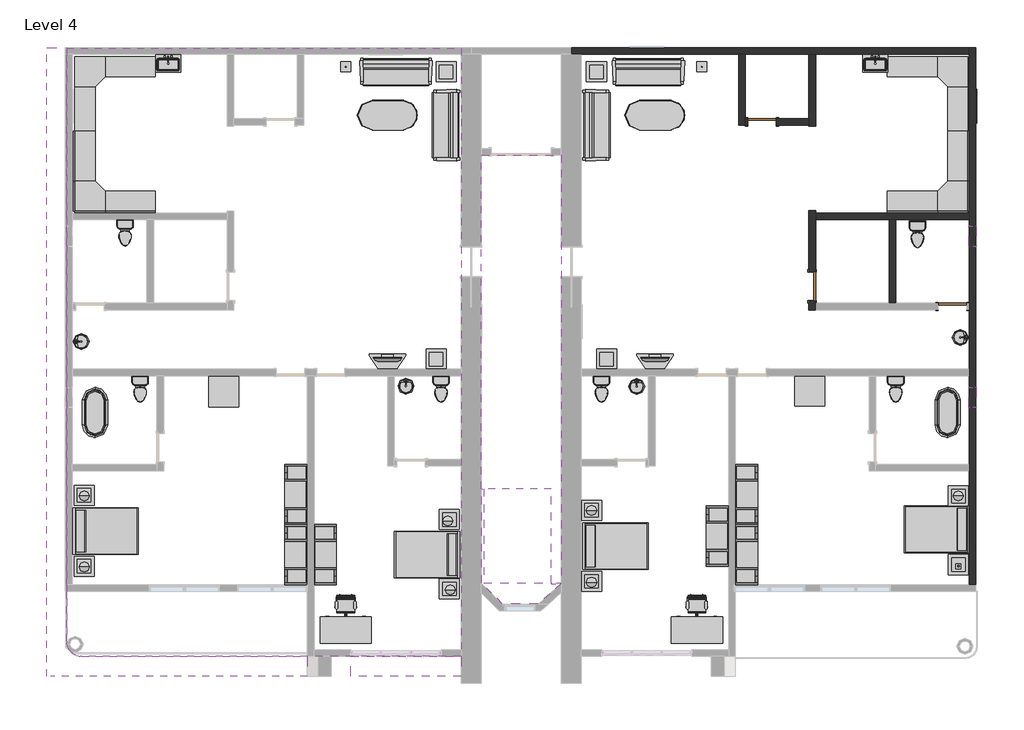
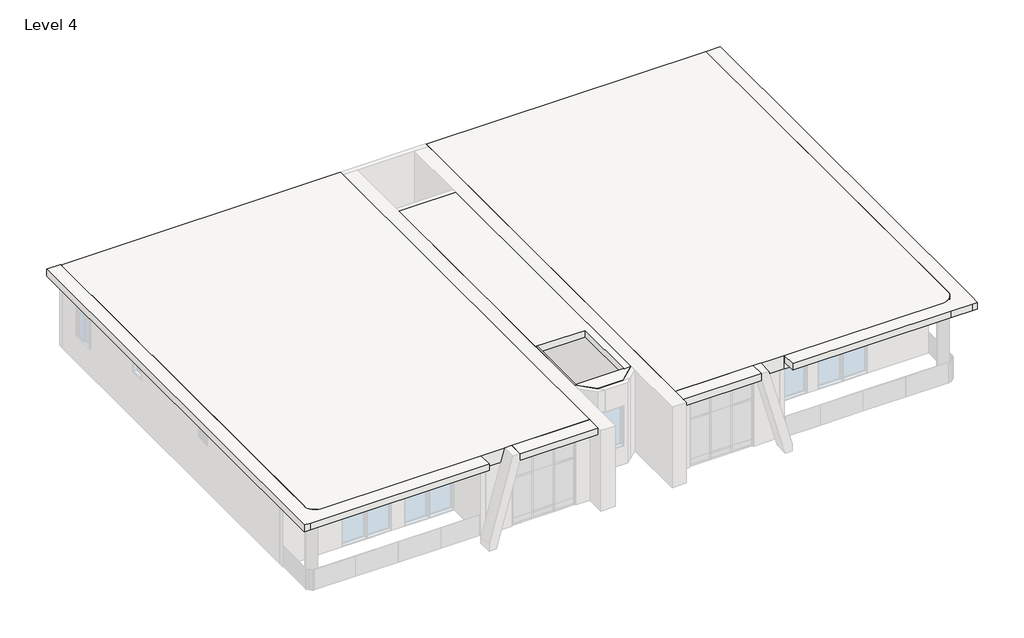
# One storey, part 3 of 3: 42 furniture elements, 14 flow terminals, 10 light fixtures, 8 walls, 5 slabs, 3 doors, 3 windows.
# Revit data of these elements (continued)
# Elements 42, 43, 44, 45, 46, 47, 48, 49, 50, 51, 52, 53 (IfcFurniture, "Table-Coffee : 24\" x 24\" x 24\"")
#   Phase Created = New Construction
#   Materials on its faces: "Glass - Clear, Grey"
# Elements 54, 55 (IfcFurniture, "Table-Dining Oval : 36\" x 72\"")
#   Phase Created = New Construction
#   Materials on its faces: "Steel, Chrome Plated", "Glass - Clear, Grey"
# Elements 56, 57 (IfcFurniture, "Table-Rectangular : 36\" x 36\"")
#   Phase Created = New Construction
#   Materials on its faces: "Birch"
# Elements 58, 59 (IfcFurniture, "Work Station Cubicle : 96\" x 96\"")
#   Phase Created = New Construction
#   Materials on its faces: "Textile - Light Gray", "Laminate, Ivory, Matte"
# Element 60 (IfcLightFixture, "100W - 120V")
#   Mark = "54"
#   Phase Created = New Construction
#   Materials on its faces: "Steel, Chrome Plated", "Glass, Frosted"
# Element 61 (IfcLightFixture, "100W - 120V")
#   Mark = "55"
#   Phase Created = New Construction
#   Materials on its faces: "Steel, Chrome Plated", "Glass, Frosted"
# Element 62 (IfcLightFixture, "Table Lamp - Hemispheric : 60W - 120V")
#   Mark = "56"
#   Phase Created = New Construction
#   Materials on its faces: "Steel, Chrome Plated", "Glass, Frosted", "Birch"
# Element 63 (IfcLightFixture, "Table Lamp - Hemispheric : 60W - 120V")
#   Mark = "57"
#   Phase Created = New Construction
#   Materials on its faces: "Steel, Chrome Plated", "Glass, Frosted", "Birch"
# Element 64 (IfcLightFixture, "Table Lamp - Hemispheric : 60W - 120V")
#   Mark = "58"
#   Phase Created = New Construction
#   Materials on its faces: "Steel, Chrome Plated", "Glass, Frosted", "Birch"
# Element 65 (IfcLightFixture, "Table Lamp - Hemispheric : 60W - 120V")
#   Mark = "59"
#   Phase Created = New Construction
#   Materials on its faces: "Steel, Chrome Plated", "Glass, Frosted", "Birch"
# Element 66 (IfcLightFixture, "Table Lamp - Hemispheric : 60W - 120V")
#   Mark = "60"
#   Phase Created = New Construction
#   Materials on its faces: "Steel, Chrome Plated", "Glass, Frosted", "Birch"
# Element 67 (IfcLightFixture, "Table Lamp - Hemispheric : 60W - 120V")
#   Mark = "61"
#   Phase Created = New Construction
#   Materials on its faces: "Steel, Chrome Plated", "Glass, Frosted", "Birch"
# Element 68 (IfcLightFixture, "Table Lamp - Hemispheric : 60W - 120V")
#   Mark = "62"
#   Phase Created = New Construction
#   Materials on its faces: "Steel, Chrome Plated", "Glass, Frosted", "Birch"
# Element 69 (IfcLightFixture, "Table Lamp - Hemispheric : 60W - 120V")
#   Mark = "63"
#   Phase Created = New Construction
#   Materials on its faces: "Steel, Chrome Plated", "Glass, Frosted", "Birch"
# Element 70 (IfcSlab, "Generic - 12\" cream")
#   Height Offset From Level = 12' - 0"
#   Phase Created = New Construction
#   Materials on its faces: "Parking Stripe"
# Element 71 (IfcSlab, "Generic - 12\" white")
#   built-in parameter 1001955 = 3.14159 (stored number, unit not read)
#   Height Offset From Level = 12' - 0"
#   Phase Created = New Construction
#   Materials on its faces: "Door - Frame"
# Elements 72, 73, 74 (IfcSlab, "Generic - 12\" white")
#   Height Offset From Level = 12' - 0"
#   Phase Created = New Construction
#   Materials on its faces: "Door - Frame"
# Elements 75, 76, 77, 78, 79, 80, 81 (IfcWall, "Generic - 8\" cream")
#   Top Offset = 0' - 0"
#   Base Offset = 0' - 0"
#   Unconnected Height = 10' - 0"
#   wall height = 10' - 0"
#   Phase Created = New Construction
#   Base Constraint = Level 4
#   Materials on its faces: "Parking Stripe"
# Element 82 (IfcWall, "Generic - 8\" white")
#   Top Offset = 0' - 0"
#   Base Offset = 0' - 0"
#   Unconnected Height = 10' - 0"
#   wall height = 10' - 0"
#   Phase Created = New Construction
#   Base Constraint = Level 4
#   Materials on its faces: "Door - Frame", "Parking Stripe"
# Element 83 (IfcWindow, "Louvers with Trim : 24\" x 24\"")
#   Mark = "110"
#   Phase Created = New Construction
#   Materials on its faces: "Glass", "Iron, Ductile"
# Element 84 (IfcWindow, "Louvers with Trim : 24\" x 24\"")
#   Mark = "111"
#   Phase Created = New Construction
#   Materials on its faces: "Glass", "Iron, Ductile"
# Element 85 (IfcWindow, "Slider with Trim : 36\" x 48\"")
#   Mark = "107"
#   Phase Created = New Construction
#   Materials on its faces: "Iron, Ductile", "Glass"
# Materials
#   "Wood - Birch - Solid Stained Light Low Gloss": class "Wood", colour RGB 210 159 95, transparency 0, Cost = 0
#   "Paint - Sienna": colour RGB 118 70 51, transparency 0, Cost = 0
#   "Steel, Polished": class "Metal", colour RGB 57 57 57, transparency 0, Description = "Polished steel", Cost = 0
#   "Porcelain, Linen": class "Ceramic", colour RGB 249 239 230, transparency 0, Description = "Porcelain, linen", Cost = 0
#   "Laminate, Linen, Matte": class "Plastic", colour RGB 249 239 230, transparency 0, Description = "Plastic Laminate - Linen, Matte", Cost = 0
#   "Porcelain, Ivory": class "Ceramic", colour RGB 247 247 239, transparency 0, Description = "Porcelain, ivory", Cost = 0
#   "Laminate, Ivory, Matte": class "Plastic", colour RGB 247 247 239, transparency 0, Description = "Plastic Laminate - Ivory, Matte", Cost = 0
#   "Birch": class "Wood", colour RGB 224 178 126, transparency 0, Description = "Betula Alleghaniensis", Cost = 0
#   "Linen, White": class "Textile", colour RGB 247 247 239, transparency 0, Description = "Linen, white", Cost = 0
#   "Plastic, Opaque Black": class "Plastic", colour RGB 0 0 0, transparency 0.7, Description = "Plastic, generic, opaque black", Cost = 0
#   "Textile - Slate Blue": class "Fabric", colour RGB 98 102 118, transparency 0
#   "Steel, Chrome Plated": class "Metal", colour RGB 17 17 17, transparency 0, Description = "Chromiuim plated steel", Cost = 0
#   "Cherry": class "Wood", colour RGB 226 177 128, transparency 0, Description = "Prunus Serotina", Cost = 0
#   "Linen, Beige": class "Textile", colour RGB 249 239 230, transparency 0, Description = "Linen, beige", Cost = 0
#   "Melamine - Gray": class "Wood", colour RGB 49 49 49, transparency 0
#   "Glass - Clear, Grey": class "Glass", colour RGB 252 255 255, transparency 0.64
#   "Textile - Light Gray": class "Fabric", colour RGB 204 204 204, transparency 0
#   "Glass, Frosted": class "Glass", colour RGB 250 244 225, transparency 0.55, Description = "physical material", Cost = 0
#   "Parking Stripe": class "Paint", colour RGB 250 250 91, transparency 0, Cost = 0
#   "Door - Frame": colour RGB 118 70 51, transparency 0, Cost = 0
#   "Iron, Ductile": class "Metal", colour RGB 0 0 0, transparency 0, Description = "Ductile cast iron", Cost = 0
#   "Glass": class "Glass", colour RGB 0 128 192, transparency 0.75, Description = "Soda Lime Glass", Cost = 0
#   "TV - Black": colour RGB 49 49 49, transparency 0
#   "TV - Glass": colour RGB 157 157 157, transparency 0.9
#   "TV - Screen": colour RGB 0 0 0, transparency 0
#   "Glass - Shelves": class "Glass", colour RGB 167 167 167, transparency 0.9
